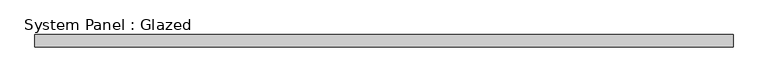
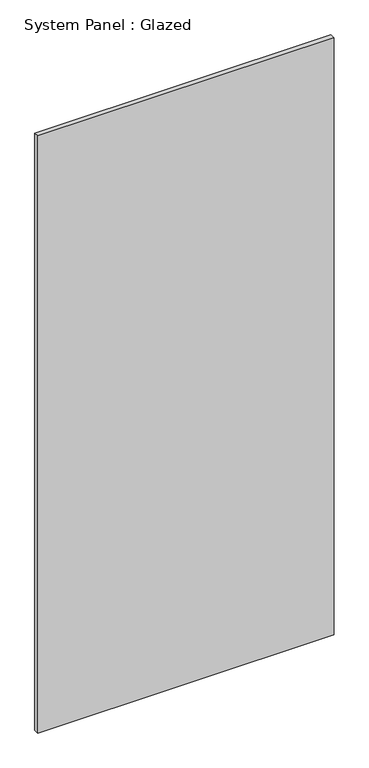
"""IFC4 building model written with IfcOpenShell, lengths in millimetres: plate geometry, System Panel : Glazed."""

from ifc_helpers import new_model, si_unit, origin, origin_with_axes, place, context, project, spatial, polyline, outline, extrude, source, transform, mapped, element, save


def system_panel_glazed_1575378d(model_context):
    return source(origin(), model_context, "Body", "SweptSolid", [
        extrude(outline(polyline([(715.1143256, 24.5), (-715.1143256, 24.5), (-715.1143256, 49.5), (715.1143256, 49.5), (715.1143256, 24.5)])), origin_with_axes(), (0.0, 0.0, 1.0), 3048.0),
    ])


if __name__ == "__main__":
    model = new_model("IFC4")
    model_context = context("Model", 3, world=origin())
    ifc_project = project(units=[si_unit("LENGTHUNIT", "METRE", prefix="MILLI")], contexts=[model_context])
    site = spatial("IfcSite", under=ifc_project)
    building = spatial("IfcBuilding", under=site)
    placement = place(None, origin())
    system_panel_glazed_shape = system_panel_glazed_1575378d(model_context)
    element("IfcPlate", 1, ObjectType="System Panel : Glazed", at=placement, inside=building, context=model_context, shape_type="MappedRepresentation", body=[
        mapped(system_panel_glazed_shape, transform((0.0, 0.0, 0.0), x_axis=(1.0, 0.0, 0.0), y_axis=(0.0, 1.0, 0.0), z_axis=(0.0, 0.0, 1.0))),
    ])
    save(model, "model.ifc")

# Revit data of these elements
# Type "System Panel : Glazed"
#   Keynote = "H11"
#   Construction Type Id = "GSP4R"
#   Analytic Construction = "1/8 in Pilkington single glazing"
#   Visual Light Transmittance = 0.9
#   Solar Heat Gain Coefficient = 0.86
#   Heat Transfer Coefficient (U) = 6.7069 W/(m²·K)
#   Define Thermal Properties by = 1
# Element 1 (IfcPlate, "System Panel : Glazed")
#   Materials on its faces: "Glass"
# Materials
#   "Glass": class "Glass", colour RGB 0 128 192, transparency 0.9, Description = "Soda Lime Glass", Cost = 0
